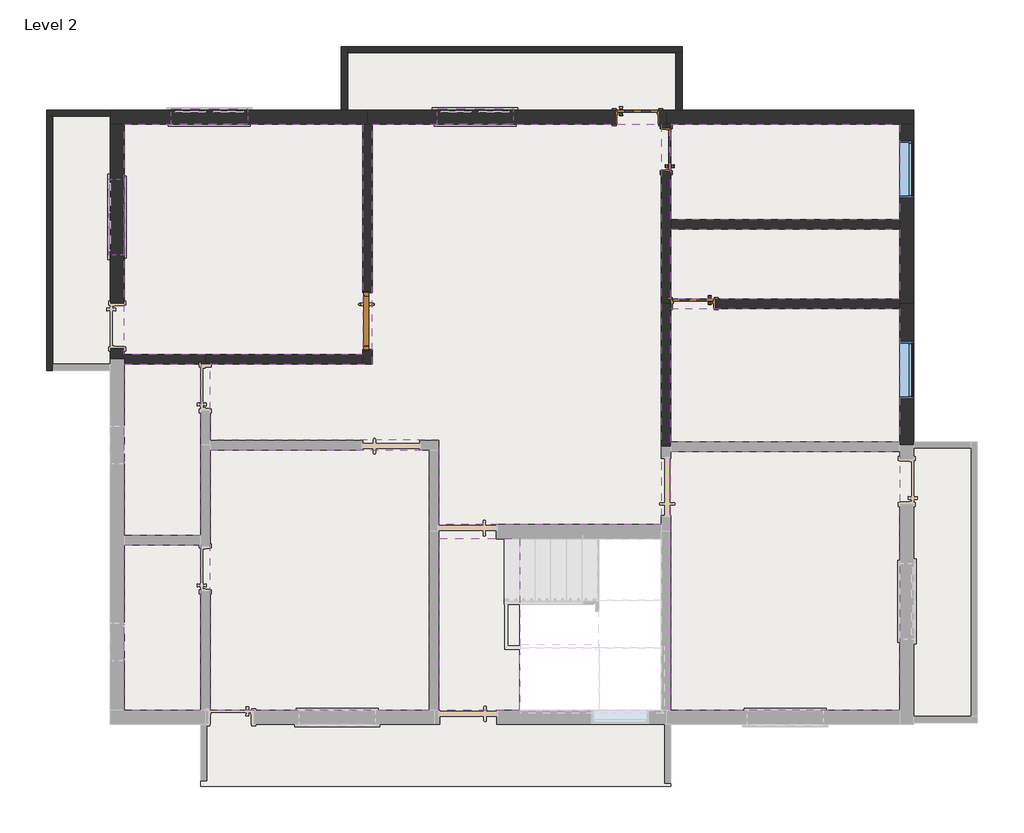
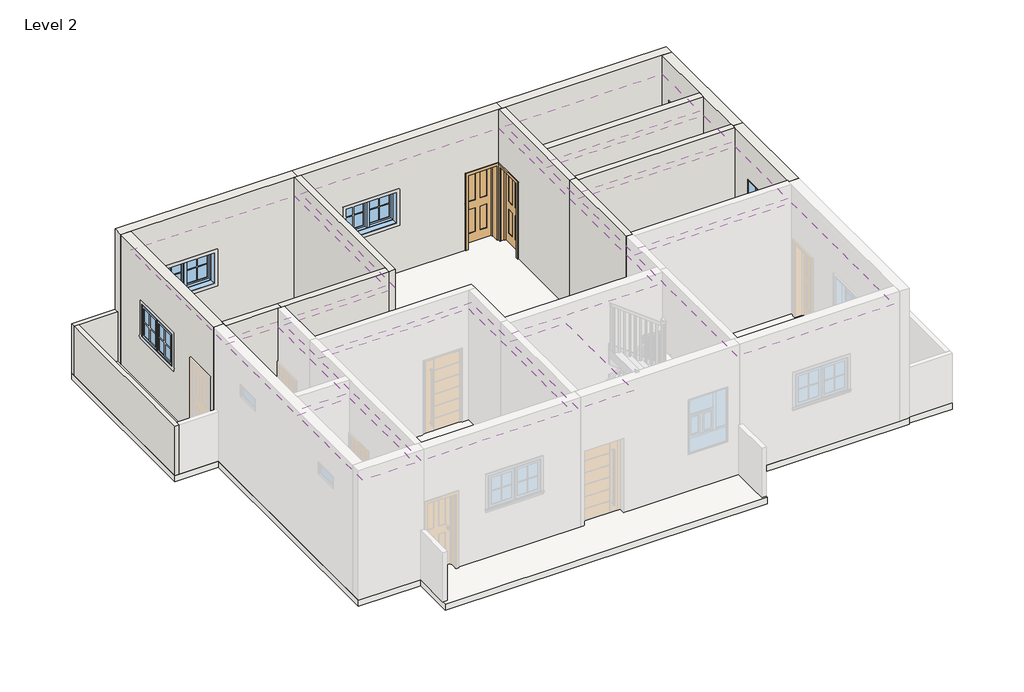
# One storey, part 2 of 3: 18 walls, 10 coverings, 5 windows, 4 doors, 1 slab.
"""IFC4 building model written with IfcOpenShell, lengths in millimetres."""

from ifc_helpers import new_model, si_unit, frame, origin, place, context, project, spatial, polyline, outline, extrude, faceted_brep, transform, mapped, element, save
from components import door_3_44036f4b, door_7109d6db, door_46909e31, m_window_awning_double_horizontal_4_8afcb0b2, m_window_casement_double_sash_variable_3_661e274a

model = new_model("IFC4")

# Units and contexts
model_context = context("Model", 3, world=origin())
ifc_project = project(units=[si_unit("LENGTHUNIT", "METRE", prefix="MILLI")], contexts=[model_context])

# Site, building, storey
site = spatial("IfcSite", under=ifc_project)
building = spatial("IfcBuilding", under=site)
storey = spatial("IfcBuildingStorey", under=building, Name="Level 2", Elevation=3200.4)

# Coverings
placement = place(None, origin())
element("IfcCovering", 1, ObjectType="Plain", at=placement, inside=storey, context=model_context, shape_type="SweptSolid", body=[
    extrude(outline(polyline([(-18062.7794909, 5121.4381491), (-14252.7794909, 5121.4381491), (-14252.7794909, 1438.4381491), (-16767.3794909, 1438.4381491), (-18062.7794909, 1438.4381491), (-18062.7794909, 5121.4381491)])), frame((0.0, 0.0, 5943.6), z_axis=(0.0, 0.0, 1.0), x_axis=(1.0, 0.0, 0.0)), (0.0, 0.0, 1.0), 57.0),
])
element("IfcCovering", 2, ObjectType="Plain", at=placement, inside=storey, context=model_context, shape_type="SweptSolid", body=[
    extrude(outline(polyline([(-16691.1794909, 1286.0381491), (-14100.3794909, 1286.0381491), (-14100.3794909, 5121.4381491), (-9477.5794909, 5121.4381491), (-9477.5794909, 2251.2381491), (-9477.5794909, -34.7618509), (-9477.5794909, -1279.3618509), (-13033.5794909, -1279.3618509), (-13033.5794909, 66.8381491), (-16691.1794909, 66.8381491), (-16691.1794909, 1286.0381491)])), frame((0.0, 0.0, 5943.6), z_axis=(0.0, 0.0, 1.0), x_axis=(1.0, 0.0, 0.0)), (0.0, 0.0, 1.0), 57.0),
])
element("IfcCovering", 3, ObjectType="Plain", at=placement, inside=storey, context=model_context, shape_type="SweptSolid", body=[
    extrude(outline(polyline([(-16843.5794909, -1457.1618509), (-18062.7794909, -1457.1618509), (-18062.7794909, 1286.0381491), (-16843.5794909, 1286.0381491), (-16843.5794909, -9.3618509), (-16843.5794909, -1457.1618509)])), frame((0.0, 0.0, 5943.6), z_axis=(0.0, 0.0, 1.0), x_axis=(1.0, 0.0, 0.0)), (0.0, 0.0, 1.0), 57.0),
])
element("IfcCovering", 4, ObjectType="Plain", at=placement, inside=storey, context=model_context, shape_type="SweptSolid", body=[
    extrude(outline(polyline([(-18062.7794909, -4251.1618509), (-18062.7794909, -1609.5618509), (-16843.5794909, -1609.5618509), (-16843.5794909, -4251.1618509), (-18062.7794909, -4251.1618509)])), frame((0.0, 0.0, 5943.6), z_axis=(0.0, 0.0, 1.0), x_axis=(1.0, 0.0, 0.0)), (0.0, 0.0, 1.0), 57.0),
])
element("IfcCovering", 5, ObjectType="Plain", at=placement, inside=storey, context=model_context, shape_type="SweptSolid", body=[
    extrude(outline(polyline([(-16691.1794909, -4251.1618509), (-16691.1794909, -85.5618509), (-13185.9794909, -85.5618509), (-13185.9794909, -1393.6618509), (-13185.9794909, -4251.1618509), (-16691.1794909, -4251.1618509)])), frame((0.0, 0.0, 5943.6), z_axis=(0.0, 0.0, 1.0), x_axis=(1.0, 0.0, 0.0)), (0.0, 0.0, 1.0), 57.0),
])
element("IfcCovering", 6, ObjectType="Plain", at=placement, inside=storey, context=model_context, shape_type="SweptSolid", body=[
    extrude(outline(polyline([(-13033.5794909, -4251.1618509), (-13033.5794909, -1507.9618509), (-11738.1794909, -1507.9618509), (-11738.1794909, -4251.1618509), (-13033.5794909, -4251.1618509)])), frame((0.0, 0.0, 5943.6), z_axis=(0.0, 0.0, 1.0), x_axis=(1.0, 0.0, 0.0)), (0.0, 0.0, 1.0), 57.0),
])
element("IfcCovering", 7, ObjectType="Plain", at=placement, inside=storey, context=model_context, shape_type="SweptSolid", body=[
    extrude(outline(polyline([(-5667.5794909, -4251.1618509), (-9325.1794909, -4251.1618509), (-9325.1794909, -1393.6618509), (-9325.1794909, -110.9618509), (-5667.5794909, -110.9618509), (-5667.5794909, -4251.1618509)])), frame((0.0, 0.0, 5943.6), z_axis=(0.0, 0.0, 1.0), x_axis=(1.0, 0.0, 0.0)), (0.0, 0.0, 1.0), 57.0),
])
element("IfcCovering", 8, ObjectType="Plain", at=placement, inside=storey, context=model_context, shape_type="SweptSolid", body=[
    extrude(outline(polyline([(-9325.1794909, 2175.0381491), (-5667.5794909, 2175.0381491), (-5667.5794909, 41.4381491), (-9325.1794909, 41.4381491), (-9325.1794909, 2175.0381491)])), frame((0.0, 0.0, 5943.6), z_axis=(0.0, 0.0, 1.0), x_axis=(1.0, 0.0, 0.0)), (0.0, 0.0, 1.0), 57.0),
])
element("IfcCovering", 9, ObjectType="Plain", at=placement, inside=storey, context=model_context, shape_type="SweptSolid", body=[
    extrude(outline(polyline([(-5667.5794909, 3445.0381491), (-5667.5794909, 2327.4381491), (-9325.1794909, 2327.4381491), (-9325.1794909, 3445.0381491), (-5667.5794909, 3445.0381491)])), frame((0.0, 0.0, 5943.6), z_axis=(0.0, 0.0, 1.0), x_axis=(1.0, 0.0, 0.0)), (0.0, 0.0, 1.0), 57.0),
])
element("IfcCovering", 10, ObjectType="Plain", at=placement, inside=storey, context=model_context, shape_type="SweptSolid", body=[
    extrude(outline(polyline([(-5667.5794909, 5121.4381491), (-5667.5794909, 3597.4381491), (-9325.1794909, 3597.4381491), (-9325.1794909, 5121.4381491), (-5667.5794909, 5121.4381491)])), frame((0.0, 0.0, 5943.6), z_axis=(0.0, 0.0, 1.0), x_axis=(1.0, 0.0, 0.0)), (0.0, 0.0, 1.0), 57.0),
])

# Doors
door_3_shape = door_3_44036f4b(model_context)
element("IfcDoor", 11, ObjectType="3'", at=placement, inside=storey, context=model_context, shape_type="MappedRepresentation", body=[
    mapped(door_3_shape, transform((-14176.5794909, 1971.8381491, 3200.4), x_axis=(0.0, -1.0, 0.0), y_axis=(1.0, 0.0, 0.0), z_axis=(0.0, 0.0, 1.0))),
])
door_shape = door_7109d6db(model_context)
element("IfcDoor", 12, ObjectType="M_Door-Interior-Single-4_Panel-Wood : 2'2\"", at=placement, inside=storey, context=model_context, shape_type="MappedRepresentation", body=[
    mapped(door_shape, transform((-9398.2044909, 4715.4381491, 3200.4), x_axis=(0.0, 1.0, 0.0), y_axis=(-1.0, 0.0, 0.0), z_axis=(0.0, 0.0, 1.0))),
])
element("IfcDoor", 13, ObjectType="M_Door-Interior-Single-4_Panel-Wood : 2'2\"", at=placement, inside=storey, context=model_context, shape_type="MappedRepresentation", body=[
    mapped(door_shape, transform((-8969.9794909, 2254.4131491, 3200.4), x_axis=(-1.0, 0.0, 0.0), y_axis=(0.0, -1.0, 0.0), z_axis=(0.0, 0.0, 1.0))),
])
door_2_shape = door_46909e31(model_context)
element("IfcDoor", 14, ObjectType="M_Door-Interior-Single-4_Panel-Wood : 2'2\"", at=placement, inside=storey, context=model_context, shape_type="MappedRepresentation", body=[
    mapped(door_2_shape, transform((-9858.1794909, 5238.9131491, 3200.4), x_axis=(1.0, 0.0, 0.0), y_axis=(0.0, 1.0, 0.0), z_axis=(0.0, 0.0, 1.0))),
])

# Slab
element("IfcSlab", 15, ObjectType="Generic 150mm", at=placement, inside=storey, context=model_context, shape_type="SweptSolid", body=[
    extrude(outline(polyline([(-18291.3794909, 1184.4381491), (-19307.3794909, 1184.4381491), (-19307.3794909, 5350.0381491), (-14596.2721539, 5350.0381491), (-14596.2721539, 6366.0381491), (-9142.3367869, 6366.0381491), (-9142.3367869, 5350.0381491), (-5438.9794909, 5350.0381491), (-5438.9794909, 41.4381491), (-4422.9794909, 41.4381491), (-4422.9794909, -4454.3618509), (-5438.9794909, -4454.3618509), (-5438.9794909, -4479.7618509), (-9325.1794909, -4479.7618509), (-9325.1794909, -5470.3618509), (-16843.5794909, -5470.3618509), (-16843.5794909, -4479.7618509), (-18291.3794909, -4479.7618509), (-18291.3794909, 1184.4381491)]), holes=[polyline([(-11738.1794909, -1507.9618509), (-11738.1794909, -4251.1618509), (-9477.5794909, -4251.1618509), (-9477.5794909, -1507.9618509), (-11738.1794909, -1507.9618509)])]), frame((0.0, 0.0, 3050.4), z_axis=(0.0, 0.0, 1.0), x_axis=(1.0, 0.0, 0.0)), (0.0, 0.0, 1.0), 150.0),
])

# Walls
element("IfcWall", 16, ObjectType="Generic - 4\"", at=placement, inside=storey, context=model_context, shape_type="Brep", body=[
    faceted_brep([(-14494.6721539, 5350.0381491, 3200.4), (-14494.6721539, 6264.4381491, 3200.4), (-14494.6721539, 6366.0381491, 3200.4), (-14494.6721539, 6366.0381491, 4419.6), (-14494.6721539, 6264.4381491, 4419.6), (-14494.6721539, 5350.0381491, 4419.6), (-14596.2721539, 5350.0381491, 3200.4), (-14596.2721539, 5350.0381491, 4419.6), (-14596.2721539, 6366.0381491, 4419.6), (-14596.2721539, 6366.0381491, 3200.4)], [[[0, 1, 2, 3, 4, 5]], [[6, 7, 8, 9]], [[2, 1, 0, 6, 9]], [[5, 4, 3, 8, 7]], [[0, 5, 7, 6]], [[3, 2, 9, 8]]]),
])
element("IfcWall", 17, ObjectType="Generic - 4\"", at=placement, inside=storey, context=model_context, shape_type="Brep", body=[
    faceted_brep([(-14494.6721539, 6264.4381491, 3200.4), (-9243.9367869, 6264.4381491, 3200.4), (-9142.3367869, 6264.4381491, 3200.4), (-9142.3367869, 6264.4381491, 4419.6), (-9243.9367869, 6264.4381491, 4419.6), (-14494.6721539, 6264.4381491, 4419.6), (-14494.6721539, 6366.0381491, 3200.4), (-14494.6721539, 6366.0381491, 4419.6), (-9142.3367869, 6366.0381491, 4419.6), (-9142.3367869, 6366.0381491, 3200.4)], [[[0, 1, 2, 3, 4, 5]], [[6, 7, 8, 9]], [[2, 1, 0, 6, 9]], [[5, 4, 3, 8, 7]], [[0, 5, 7, 6]], [[3, 2, 9, 8]]]),
])
element("IfcWall", 18, ObjectType="Generic - 4\"", at=placement, inside=storey, context=model_context, shape_type="SweptSolid", body=[
    extrude(outline(polyline([(-9243.9367869, 5350.0381491), (-9243.9367869, 6264.4381491), (-9142.3367869, 6264.4381491), (-9142.3367869, 5350.0381491), (-9243.9367869, 5350.0381491)])), frame((0.0, 0.0, 3200.4), z_axis=(0.0, 0.0, 1.0), x_axis=(1.0, 0.0, 0.0)), (0.0, 0.0, 1.0), 1219.2),
])
element("IfcWall", 19, ObjectType="Generic - 4\"", at=placement, inside=storey, context=model_context, shape_type="Brep", body=[
    faceted_brep([(-18291.3794909, 5350.0381491, 3200.4), (-19307.3794909, 5350.0381491, 3200.4), (-19307.3794909, 5350.0381491, 4419.6), (-18291.3794909, 5350.0381491, 4419.6), (-18291.3794909, 5248.4381491, 3200.4), (-18291.3794909, 5248.4381491, 4419.6), (-19205.7794909, 5248.4381491, 4419.6), (-19307.3794909, 5248.4381491, 4419.6), (-19307.3794909, 5248.4381491, 3200.4), (-19205.7794909, 5248.4381491, 3200.4)], [[[0, 1, 2, 3]], [[4, 5, 6, 7, 8, 9]], [[1, 0, 4, 9, 8]], [[3, 2, 7, 6, 5]], [[0, 3, 5, 4]], [[2, 1, 8, 7]]]),
])
element("IfcWall", 20, ObjectType="Generic - 4\"", at=placement, inside=storey, context=model_context, shape_type="Brep", body=[
    faceted_brep([(-19307.3794909, 5248.4381491, 3200.4), (-19307.3794909, 1184.4381491, 3200.4), (-19307.3794909, 1184.4381491, 4419.6), (-19307.3794909, 5248.4381491, 4419.6), (-19205.7794909, 5248.4381491, 3200.4), (-19205.7794909, 5248.4381491, 4419.6), (-19205.7794909, 1286.0381491, 4419.6), (-19205.7794909, 1184.4381491, 4419.6), (-19205.7794909, 1184.4381491, 3200.4), (-19205.7794909, 1286.0381491, 3200.4)], [[[0, 1, 2, 3]], [[4, 5, 6, 7, 8, 9]], [[1, 0, 4, 9, 8]], [[3, 2, 7, 6, 5]], [[0, 3, 5, 4]], [[2, 1, 8, 7]]]),
])
element("IfcWall", 21, ObjectType="Generic - 6\"", at=placement, inside=storey, context=model_context, shape_type="Brep", body=[
    faceted_brep([(-14252.7794909, 1286.0381491, 6400.8), (-14252.7794909, 1438.4381491, 6400.8), (-14252.7794909, 5121.4381491, 6400.8), (-14252.7794909, 5121.4381491, 3200.4), (-14252.7794909, 2429.0381491, 3200.4), (-14252.7794909, 2429.0381491, 5029.2), (-14252.7794909, 1514.6381491, 5029.2), (-14252.7794909, 1514.6381491, 3200.4), (-14252.7794909, 1438.4381491, 3200.4), (-14252.7794909, 1286.0381491, 3200.4), (-14100.3794909, 5121.4381491, 6400.8), (-14100.3794909, 1286.0381491, 6400.8), (-14100.3794909, 1286.0381491, 3200.4), (-14100.3794909, 1514.6381491, 3200.4), (-14100.3794909, 1514.6381491, 5029.2), (-14100.3794909, 2429.0381491, 5029.2), (-14100.3794909, 2429.0381491, 3200.4), (-14100.3794909, 5121.4381491, 3200.4), (-14232.7794909, 1514.6381491, 3200.4), (-14232.7794909, 1499.6381491, 3200.4), (-14155.7794909, 1499.6381491, 3200.4), (-14155.7794909, 1514.6381491, 3200.4), (-14176.5794909, 5121.4381491, 3200.4), (-14155.7794909, 2429.0381491, 3200.4), (-14155.7794909, 2444.0381491, 3200.4), (-14232.7794909, 2444.0381491, 3200.4), (-14232.7794909, 2429.0381491, 3200.4), (-14176.5794909, 5121.4381491, 6400.8), (-14232.7794909, 2429.0381491, 5029.2), (-14232.7794909, 1514.6381491, 5029.2), (-14155.7794909, 1514.6381491, 5029.2), (-14155.7794909, 2429.0381491, 5029.2), (-14232.7794909, 2444.0381491, 5044.2), (-14155.7794909, 2444.0381491, 5044.2), (-14155.7794909, 1499.6381491, 5044.2), (-14232.7794909, 1499.6381491, 5044.2)], [[[0, 1, 2, 3, 4, 5, 6, 7, 8, 9]], [[10, 11, 12, 13, 14, 15, 16, 17]], [[12, 9, 8, 7, 18, 19, 20, 21, 13]], [[3, 22, 17, 16, 23, 24, 25, 26, 4]], [[2, 1, 0, 11, 10, 27]], [[3, 2, 27, 10, 17, 22]], [[0, 9, 12, 11]], [[5, 28, 29, 6]], [[14, 30, 31, 15]], [[6, 29, 18, 7]], [[30, 14, 13, 21]], [[28, 5, 4, 26]], [[15, 31, 23, 16]], [[32, 33, 34, 35]], [[35, 34, 20, 19]], [[31, 30, 21, 20, 34, 33, 24, 23]], [[33, 32, 25, 24]], [[29, 28, 26, 25, 32, 35, 19, 18]]]),
])
element("IfcWall", 22, ObjectType="Generic - 6\"", at=placement, inside=storey, context=model_context, shape_type="Brep", body=[
    faceted_brep([(-14252.7794909, 1438.4381491, 3200.4), (-16767.3794909, 1438.4381491, 3200.4), (-16767.3794909, 1438.4381491, 6400.8), (-14252.7794909, 1438.4381491, 6400.8), (-14252.7794909, 1286.0381491, 3200.4), (-14252.7794909, 1286.0381491, 6400.8), (-16691.1794909, 1286.0381491, 6400.8), (-16767.3794909, 1286.0381491, 6400.8), (-16767.3794909, 1286.0381491, 3200.4), (-16691.1794909, 1286.0381491, 3200.4)], [[[0, 1, 2, 3]], [[4, 5, 6, 7, 8, 9]], [[1, 0, 4, 9, 8]], [[2, 1, 8, 7]], [[3, 2, 7, 6, 5]], [[0, 3, 5, 4]]]),
])
element("IfcWall", 23, ObjectType="Generic - 6\"", at=placement, inside=storey, context=model_context, shape_type="SweptSolid", body=[
    extrude(outline(polyline([(-5667.5794909, 3445.0381491), (-9325.1794909, 3445.0381491), (-9325.1794909, 3597.4381491), (-5667.5794909, 3597.4381491), (-5667.5794909, 3445.0381491)])), frame((0.0, 0.0, 3200.4), z_axis=(0.0, 0.0, 1.0), x_axis=(1.0, 0.0, 0.0)), (0.0, 0.0, 1.0), 3200.4),
])
element("IfcWall", 24, ObjectType="Generic - 6\"", at=placement, inside=storey, context=model_context, shape_type="Brep", body=[
    faceted_brep([(-9325.1794909, 2327.4381491, 6400.8), (-5667.5794909, 2327.4381491, 6400.8), (-5667.5794909, 2327.4381491, 3200.4), (-8614.7794909, 2327.4381491, 3200.4), (-8614.7794909, 2327.4381491, 5054.2), (-9325.1794909, 2327.4381491, 5054.2), (-5667.5794909, 2175.0381491, 6400.8), (-9325.1794909, 2175.0381491, 6400.8), (-9325.1794909, 2175.0381491, 5054.2), (-8614.7794909, 2175.0381491, 5054.2), (-8614.7794909, 2175.0381491, 3200.4), (-5667.5794909, 2175.0381491, 3200.4), (-5667.5794909, 2251.2381491, 3200.4), (-9325.1794909, 2251.2381491, 6400.8), (-5667.5794909, 2251.2381491, 6400.8)], [[[0, 1, 2, 3, 4, 5]], [[6, 7, 8, 9, 10, 11]], [[2, 12, 11, 10, 3]], [[1, 0, 13, 7, 6, 14]], [[2, 1, 14, 6, 11, 12]], [[7, 13, 0, 5, 8]], [[4, 9, 8, 5]], [[9, 4, 3, 10]]]),
])
element("IfcWall", 25, ObjectType="Generic - 6\"", at=placement, inside=storey, context=model_context, shape_type="Brep", body=[
    faceted_brep([(-9325.1794909, 5121.4381491, 6400.8), (-9325.1794909, 3597.4381491, 6400.8), (-9325.1794909, 3445.0381491, 6400.8), (-9325.1794909, 2327.4381491, 6400.8), (-9325.1794909, 2251.2381491, 6400.8), (-9325.1794909, 2251.2381491, 3200.4), (-9325.1794909, 3445.0381491, 3200.4), (-9325.1794909, 3597.4381491, 3200.4), (-9325.1794909, 4360.2381491, 3200.4), (-9325.1794909, 4360.2381491, 5054.2), (-9325.1794909, 5070.6381491, 5054.2), (-9325.1794909, 5070.6381491, 3200.4), (-9325.1794909, 5121.4381491, 3200.4), (-9477.5794909, 2251.2381491, 6400.8), (-9477.5794909, 5121.4381491, 6400.8), (-9477.5794909, 5121.4381491, 3200.4), (-9477.5794909, 5070.6381491, 3200.4), (-9477.5794909, 5070.6381491, 5054.2), (-9477.5794909, 4360.2381491, 5054.2), (-9477.5794909, 4360.2381491, 3200.4), (-9477.5794909, 2251.2381491, 3200.4), (-9401.3794909, 5121.4381491, 3200.4), (-9401.3794909, 5121.4381491, 6400.8)], [[[0, 1, 2, 3, 4, 5, 6, 7, 8, 9, 10, 11, 12]], [[13, 14, 15, 16, 17, 18, 19, 20]], [[15, 21, 12, 11, 16]], [[5, 20, 19, 8, 7, 6]], [[4, 3, 2, 1, 0, 22, 14, 13]], [[5, 4, 13, 20]], [[0, 12, 21, 15, 14, 22]], [[10, 17, 16, 11]], [[17, 10, 9, 18]], [[18, 9, 8, 19]]]),
])
element("IfcWall", 26, ObjectType="Generic - 6\"", at=placement, inside=storey, context=model_context, shape_type="Brep", body=[
    faceted_brep([(-9325.1794909, -34.7618509, 3200.4), (-9325.1794909, 41.4381491, 3200.4), (-9325.1794909, 2251.2381491, 3200.4), (-9325.1794909, 2251.2381491, 6400.8), (-9325.1794909, 2175.0381491, 6400.8), (-9325.1794909, 41.4381491, 6400.8), (-9325.1794909, -34.7618509, 6400.8), (-9477.5794909, -34.7618509, 3200.4), (-9477.5794909, -34.7618509, 6400.8), (-9477.5794909, 2251.2381491, 6400.8), (-9477.5794909, 2251.2381491, 3200.4)], [[[0, 1, 2, 3, 4, 5, 6]], [[7, 8, 9, 10]], [[2, 1, 0, 7, 10]], [[3, 2, 10, 9]], [[6, 5, 4, 3, 9, 8]], [[0, 6, 8, 7]]]),
])
element("IfcWall", 27, ObjectType="Generic - 6\"", at=placement, inside=storey, context=model_context, shape_type="Brep", body=[
    faceted_brep([(-16767.3794909, 1438.4381491, 3200.4), (-18062.7794909, 1438.4381491, 3200.4), (-18062.7794909, 1438.4381491, 6400.8), (-16767.3794909, 1438.4381491, 6400.8), (-16767.3794909, 1286.0381491, 3200.4), (-16767.3794909, 1286.0381491, 6400.8), (-16843.5794909, 1286.0381491, 6400.8), (-18062.7794909, 1286.0381491, 6400.8), (-18062.7794909, 1286.0381491, 3200.4), (-16843.5794909, 1286.0381491, 3200.4), (-18062.7794909, 1362.2381491, 3200.4), (-18062.7794909, 1362.2381491, 6400.8)], [[[0, 1, 2, 3]], [[4, 5, 6, 7, 8, 9]], [[1, 0, 4, 9, 8, 10]], [[3, 2, 11, 7, 6, 5]], [[0, 3, 5, 4]], [[2, 1, 10, 8, 7, 11]]]),
])
element("IfcWall", 28, ObjectType="Generic - 9\"", at=placement, inside=storey, context=model_context, shape_type="Brep", body=[
    faceted_brep([(-18291.3794909, 5121.4381491, 6400.8), (-18291.3794909, 5121.4381491, 3200.4), (-18062.7794909, 5121.4381491, 3200.4), (-14252.7794909, 5121.4381491, 3200.4), (-14176.5794909, 5121.4381491, 3200.4), (-14176.5794909, 5121.4381491, 6400.8), (-14252.7794909, 5121.4381491, 6400.8), (-18062.7794909, 5121.4381491, 6400.8), (-16094.2794909, 5121.4381491, 5219.6), (-16094.2794909, 5121.4381491, 4419.6), (-17313.4794909, 5121.4381491, 4419.6), (-17313.4794909, 5121.4381491, 5219.6), (-18291.3794909, 5350.0381491, 3200.4), (-18291.3794909, 5350.0381491, 4419.6), (-18291.3794909, 5350.0381491, 6400.8), (-14176.5794909, 5350.0381491, 6400.8), (-14176.5794909, 5350.0381491, 3200.4), (-14494.6721539, 5350.0381491, 3200.4), (-14596.2721539, 5350.0381491, 3200.4), (-16094.2794909, 5350.0381491, 5219.6), (-17313.4794909, 5350.0381491, 5219.6), (-17313.4794909, 5350.0381491, 4419.6), (-16094.2794909, 5350.0381491, 4419.6), (-18291.3794909, 5248.4381491, 3200.4)], [[[0, 1, 2, 3, 4, 5, 6, 7], [8, 9, 10, 11]], [[12, 13, 14, 15, 16, 17, 18], [19, 20, 21, 22]], [[4, 3, 2, 1, 23, 12, 18, 17, 16]], [[5, 4, 16, 15]], [[0, 7, 6, 5, 15, 14]], [[0, 14, 13, 12, 23, 1]], [[9, 8, 19, 22]], [[10, 9, 22, 21]], [[11, 10, 21, 20]], [[8, 11, 20, 19]]]),
])
element("IfcWall", 29, ObjectType="Generic - 9\"", at=placement, inside=storey, context=model_context, shape_type="Brep", body=[
    faceted_brep([(-5667.5794909, 5121.4381491, 3200.4), (-5667.5794909, 3597.4381491, 3200.4), (-5667.5794909, 3445.0381491, 3200.4), (-5667.5794909, 2327.4381491, 3200.4), (-5667.5794909, 2251.2381491, 3200.4), (-5667.5794909, 2251.2381491, 6400.8), (-5667.5794909, 2327.4381491, 6400.8), (-5667.5794909, 3445.0381491, 6400.8), (-5667.5794909, 3597.4381491, 6400.8), (-5667.5794909, 5121.4381491, 6400.8), (-5667.5794909, 3943.5131491, 5450.4), (-5667.5794909, 3943.5131491, 4100.4), (-5667.5794909, 4857.9131491, 4100.4), (-5667.5794909, 4857.9131491, 5450.4), (-5438.9794909, 5121.4381491, 3200.4), (-5438.9794909, 5121.4381491, 6400.8), (-5438.9794909, 2251.2381491, 6400.8), (-5438.9794909, 2251.2381491, 3200.4), (-5438.9794909, 3943.5131491, 5450.4), (-5438.9794909, 4857.9131491, 5450.4), (-5438.9794909, 4857.9131491, 4100.4), (-5438.9794909, 3943.5131491, 4100.4)], [[[0, 1, 2, 3, 4, 5, 6, 7, 8, 9], [10, 11, 12, 13]], [[14, 15, 16, 17], [18, 19, 20, 21]], [[4, 3, 2, 1, 0, 14, 17]], [[5, 4, 17, 16]], [[9, 8, 7, 6, 5, 16, 15]], [[0, 9, 15, 14]], [[11, 10, 18, 21]], [[12, 11, 21, 20]], [[13, 12, 20, 19]], [[10, 13, 19, 18]]]),
])
element("IfcWall", 30, ObjectType="Generic - 9\"", at=placement, inside=storey, context=model_context, shape_type="Brep", body=[
    faceted_brep([(-9401.3794909, 5121.4381491, 3200.4), (-9401.3794909, 5121.4381491, 6400.8), (-9477.5794909, 5121.4381491, 6400.8), (-14100.3794909, 5121.4381491, 6400.8), (-14176.5794909, 5121.4381491, 6400.8), (-14176.5794909, 5121.4381491, 3200.4), (-14100.3794909, 5121.4381491, 3200.4), (-10213.3794909, 5121.4381491, 3200.4), (-10213.3794909, 5121.4381491, 5054.2), (-9502.9794909, 5121.4381491, 5054.2), (-9502.9794909, 5121.4381491, 3200.4), (-9477.5794909, 5121.4381491, 3200.4), (-11844.5419909, 5121.4381491, 5219.6), (-11844.5419909, 5121.4381491, 4419.6), (-13063.7419909, 5121.4381491, 4419.6), (-13063.7419909, 5121.4381491, 5219.6), (-9401.3794909, 5350.0381491, 6400.8), (-9401.3794909, 5350.0381491, 3200.4), (-9502.9794909, 5350.0381491, 3200.4), (-9502.9794909, 5350.0381491, 5054.2), (-10213.3794909, 5350.0381491, 5054.2), (-10213.3794909, 5350.0381491, 3200.4), (-14176.5794909, 5350.0381491, 3200.4), (-14176.5794909, 5350.0381491, 6400.8), (-11844.5419909, 5350.0381491, 5219.6), (-13063.7419909, 5350.0381491, 5219.6), (-13063.7419909, 5350.0381491, 4419.6), (-11844.5419909, 5350.0381491, 4419.6)], [[[0, 1, 2, 3, 4, 5, 6, 7, 8, 9, 10, 11], [12, 13, 14, 15]], [[16, 17, 18, 19, 20, 21, 22, 23], [24, 25, 26, 27]], [[5, 22, 21, 7, 6]], [[17, 0, 11, 10, 18]], [[1, 0, 17, 16]], [[4, 3, 2, 1, 16, 23]], [[5, 4, 23, 22]], [[12, 15, 25, 24]], [[15, 14, 26, 25]], [[14, 13, 27, 26]], [[13, 12, 24, 27]], [[9, 19, 18, 10]], [[19, 9, 8, 20]], [[20, 8, 7, 21]]]),
])
element("IfcWall", 31, ObjectType="Generic - 9\"", at=placement, inside=storey, context=model_context, shape_type="Brep", body=[
    faceted_brep([(-9401.3794909, 5121.4381491, 3200.4), (-9325.1794909, 5121.4381491, 3200.4), (-5667.5794909, 5121.4381491, 3200.4), (-5438.9794909, 5121.4381491, 3200.4), (-5438.9794909, 5121.4381491, 6400.8), (-5667.5794909, 5121.4381491, 6400.8), (-9325.1794909, 5121.4381491, 6400.8), (-9401.3794909, 5121.4381491, 6400.8), (-9401.3794909, 5350.0381491, 3200.4), (-9401.3794909, 5350.0381491, 6400.8), (-5438.9794909, 5350.0381491, 6400.8), (-5438.9794909, 5350.0381491, 3200.4), (-9142.3367869, 5350.0381491, 3200.4), (-9243.9367869, 5350.0381491, 3200.4)], [[[0, 1, 2, 3, 4, 5, 6, 7]], [[8, 9, 10, 11, 12, 13]], [[3, 2, 1, 0, 8, 13, 12, 11]], [[7, 6, 5, 4, 10, 9]], [[0, 7, 9, 8]], [[4, 3, 11, 10]]]),
])
element("IfcWall", 32, ObjectType="Generic - 9\"", at=placement, inside=storey, context=model_context, shape_type="Brep", body=[
    faceted_brep([(-5667.5794909, 2251.2381491, 3200.4), (-5667.5794909, 2175.0381491, 3200.4), (-5667.5794909, -9.3618509, 3200.4), (-5667.5794909, -9.3618509, 6400.8), (-5667.5794909, 2175.0381491, 6400.8), (-5667.5794909, 2251.2381491, 6400.8), (-5667.5794909, 732.0006491, 5450.4), (-5667.5794909, 732.0006491, 4100.4), (-5667.5794909, 1646.4006491, 4100.4), (-5667.5794909, 1646.4006491, 5450.4), (-5438.9794909, 2251.2381491, 3200.4), (-5438.9794909, 2251.2381491, 6400.8), (-5438.9794909, -9.3618509, 6400.8), (-5438.9794909, -9.3618509, 3200.4), (-5438.9794909, 41.4381491, 3200.4), (-5438.9794909, 732.0006491, 5450.4), (-5438.9794909, 1646.4006491, 5450.4), (-5438.9794909, 1646.4006491, 4100.4), (-5438.9794909, 732.0006491, 4100.4)], [[[0, 1, 2, 3, 4, 5], [6, 7, 8, 9]], [[10, 11, 12, 13, 14], [15, 16, 17, 18]], [[2, 1, 0, 10, 14, 13]], [[5, 4, 3, 12, 11]], [[0, 5, 11, 10]], [[6, 9, 16, 15]], [[9, 8, 17, 16]], [[8, 7, 18, 17]], [[7, 6, 15, 18]], [[2, 13, 12, 3]]]),
])
element("IfcWall", 33, ObjectType="Generic - 9\"", at=placement, inside=storey, context=model_context, shape_type="Brep", body=[
    faceted_brep([(-18062.7794909, 5121.4381491, 6400.8), (-18062.7794909, 1438.4381491, 6400.8), (-18062.7794909, 1362.2381491, 6400.8), (-18062.7794909, 1362.2381491, 3200.4), (-18062.7794909, 1438.4381491, 3200.4), (-18062.7794909, 1540.0381491, 3200.4), (-18062.7794909, 1540.0381491, 5054.2), (-18062.7794909, 2250.4381491, 5054.2), (-18062.7794909, 2250.4381491, 3200.4), (-18062.7794909, 5121.4381491, 3200.4), (-18062.7794909, 4247.5131491, 5219.6), (-18062.7794909, 4247.5131491, 4419.6), (-18062.7794909, 3028.3131491, 4419.6), (-18062.7794909, 3028.3131491, 5219.6), (-18291.3794909, 1362.2381491, 6400.8), (-18291.3794909, 5121.4381491, 6400.8), (-18291.3794909, 5121.4381491, 3200.4), (-18291.3794909, 2250.4381491, 3200.4), (-18291.3794909, 2250.4381491, 5054.2), (-18291.3794909, 1540.0381491, 5054.2), (-18291.3794909, 1540.0381491, 3200.4), (-18291.3794909, 1362.2381491, 3200.4), (-18291.3794909, 4247.5131491, 5219.6), (-18291.3794909, 3028.3131491, 5219.6), (-18291.3794909, 3028.3131491, 4419.6), (-18291.3794909, 4247.5131491, 4419.6)], [[[0, 1, 2, 3, 4, 5, 6, 7, 8, 9], [10, 11, 12, 13]], [[14, 15, 16, 17, 18, 19, 20, 21], [22, 23, 24, 25]], [[16, 9, 8, 17]], [[3, 21, 20, 5, 4]], [[2, 1, 0, 15, 14]], [[3, 2, 14, 21]], [[9, 16, 15, 0]], [[10, 13, 23, 22]], [[13, 12, 24, 23]], [[12, 11, 25, 24]], [[11, 10, 22, 25]], [[19, 6, 5, 20]], [[6, 19, 18, 7]], [[7, 18, 17, 8]]]),
])

# Windows
m_window_awning_double_horizontal_4_shape = m_window_awning_double_horizontal_4_8afcb0b2(model_context)
element("IfcWindow", 34, ObjectType="M_Window-Awning-Double-Horizontal : 4'", at=placement, inside=storey, context=model_context, shape_type="MappedRepresentation", body=[
    mapped(m_window_awning_double_horizontal_4_shape, transform((-16703.8794909, 5235.7381491, 3519.6), x_axis=(1.0, 0.0, 0.0), y_axis=(0.0, 1.0, 0.0), z_axis=(0.0, 0.0, 1.0))),
])
element("IfcWindow", 35, ObjectType="M_Window-Awning-Double-Horizontal : 4'", at=placement, inside=storey, context=model_context, shape_type="MappedRepresentation", body=[
    mapped(m_window_awning_double_horizontal_4_shape, transform((-18177.0794909, 3637.9131491, 3519.6), x_axis=(0.0, 1.0, 0.0), y_axis=(-1.0, 0.0, 0.0), z_axis=(0.0, 0.0, 1.0))),
])
element("IfcWindow", 36, ObjectType="M_Window-Awning-Double-Horizontal : 4'", at=placement, inside=storey, context=model_context, shape_type="MappedRepresentation", body=[
    mapped(m_window_awning_double_horizontal_4_shape, transform((-12454.1419909, 5235.7381491, 3519.6), x_axis=(1.0, 0.0, 0.0), y_axis=(0.0, 1.0, 0.0), z_axis=(0.0, 0.0, 1.0))),
])
m_window_casement_double_sash_variable_3_shape = m_window_casement_double_sash_variable_3_661e274a(model_context)
element("IfcWindow", 37, ObjectType="M_Window-Casement-Double-Sash-Variable : 3'", at=placement, inside=storey, context=model_context, shape_type="MappedRepresentation", body=[
    mapped(m_window_casement_double_sash_variable_3_shape, transform((-5553.2794909, 1189.2006491, 3200.4), x_axis=(0.0, -1.0, 0.0), y_axis=(1.0, 0.0, 0.0), z_axis=(0.0, 0.0, 1.0))),
])
element("IfcWindow", 38, ObjectType="M_Window-Casement-Double-Sash-Variable : 3'", at=placement, inside=storey, context=model_context, shape_type="MappedRepresentation", body=[
    mapped(m_window_casement_double_sash_variable_3_shape, transform((-5553.2794909, 4400.7131491, 3200.4), x_axis=(0.0, -1.0, 0.0), y_axis=(1.0, 0.0, 0.0), z_axis=(0.0, 0.0, 1.0))),
])

save(model, "model.ifc")

# Revit data of these elements
# Type "Plain"
#   built-in parameter 1002203 = 1 (stored number, unit not read)
#   built-in parameter 1002202 = 1 (stored number, unit not read)
#   Layers, outside or top first: 0' - 1.77165" "Metal Stud Layer" (function 1); 0' - 0.47244" "Gypsum Wall Board" (function 1)
# Type "3'"
#   Type Mark = "41"
#   Water resistance = "up to Class E900, EN 12208:2001"
#   Uniclass2015Version = "v1.21"
#   Uniclass2015Reference = "Ss_25_30_20_30"
#   Uniclass2015Description = "Frame and door leaf system"
#   URL = "www.aluprof.com"
#   Type IFC Predefined Type = "USERDEFINED"
#   Right-hand / Left-hand door [instance default] = ""
#   Resistance to wind load = "up to Class C5/B5, EN 12210:2001"
#   Insert type = "ST"
#   Hardware [instance default] = ""
#   Product page = "https://aluprof.com/en/architects/offer/window-and-door-systems/panel-doors#visualisation"
#   Operation = "SinglePanelOutwardOpening"
#   Opening type = "Outward"
#   NBSReference = "25-50-20/125"
#   NBSDescription = "Frame and door leaf system"
#   Important = "The actual acceptable construction dimensions are dependent on the selection of profiles and hardware, glazing type, construction weight and the construction’s operating conditions. These should be determined by a suitably qualified person, and using ALUPROF’s calculation software"
#   IfcExportType = "USERDEFINED"
#   IfcExportAs = "IfcDoorType"
#   Handle type [instance default] = ""
#   Manufacturer = "ALUPROF SA"
#   Export Type to IFC As = "IfcDoorType"
#   Door sill type [instance default] = ""
#   Description = "External single-leaf panel door outward opening"
#   Model = "MB-86 ST Panel Door AD07"
#   Content of the recyclate in the material = "69.2%"
#   COBie.Type.WarrantyDurationParts = ""
#   COBie.Type.Name = ""
#   COBie.Type.Manufacturer = "ALUPROF SA"
#   COBie.Space.Name = ""
#   COBie.Floor.Name = ""
#   COBie.Facility.Name = ""
#   COBie.CreatedOn = ""
#   COBie.Component.WarrantyStartDate = ""
#   COBie.Component.Name = "MB-86 ST Panel Door AD07"
#   Burglar resistance = "RC2"
#   Air permeability = "up to Class 4, EN 12207:2001"
#   Width of the active leaf = 2' - 8.17717"
#   Placement in wall = 0' - 0.7874"
#   Thickness = 0' - 3.0315"
#   Height of the opening sash = 5' - 9.44094"
#   Handle Offset = 3' - 5.33858"
#   Rough Height = 6' - 2.40945"
#   Rough Width = 3' - 1.1811"
#   Height = 6' - 0"
#   Width = 3' - 0"
#   Construction depth = 0' - 3.0315"
#   Clear opening width = 2' - 3.94882"
#   Clear opening height = 5' - 8.47638"
#   Height of the array = 0' - 11.08136"
#   Schedule No. [instance default] = 1
#   Handrail [instance default] = yes
#   IsExternal = yes
#   Handle [instance default] = no
#   Door closer [instance default] = no
#   Function = 1
#   COBie.Type = yes
#   COBie = yes
#   Access control [instance default] = no
#   Panel = element 361060
#   Wall Closure = (empty or 0)
# Type "M_Door-Interior-Single-4_Panel-Wood : 2'2\""
#   Type Mark = "43"
#   Assembly Code = "C1020300"
#   Analytic Construction = "Wooden"
#   Top Rail = 0' - 4.72441"
#   Thickness = 0' - 1.37795"
#   Thermal Resistance (R) = 0.455703 (m²·K)/W
#   Swing Angle [instance default] = 90.00°
#   Stiles = 0' - 4.72441"
#   Rough Width = 2' - 3.9685"
#   Rough Height = 6' - 0.98425"
#   Mullion = 0' - 4.52756"
#   Lock Rail = 0' - 7.87402"
#   Height = 6' - 0"
#   Width = 2' - 2"
#   Heat Transfer Coefficient (U) = 2.19465 W/(m²·K)
#   Bottom Rail = 0' - 9.05512"
#   Trim Material = Cherry
#   Panel Material = Cherry
#   Frame Material = Cherry
#   Door Handle Material = Aluminum
#   Visual Light Transmittance = 0
#   Solar Heat Gain Coefficient = 0
#   Wall Closure = (empty or 0)
#   Function = (empty or 0)
# Type "Generic 150mm"
#   Function = 0
#   Layers, outside or top first: 0' - 5.90551" no material (function 1)
# Type "Generic - 4\""
#   Layers, outside or top first: 0' - 4" no material (function 1)
# Type "Generic - 6\""
#   Layers, outside or top first: 0' - 6" no material (function 1)
# Type "Generic - 9\""
#   Layers, outside or top first: 0' - 9" no material (function 1)
# Type "M_Window-Awning-Double-Horizontal : 4'"
#   Type Mark = "28"
#   Fire Rating = "0.5h"
#   Assembly Code = "B2020100"
#   Analytic Construction = "Double glazing - domestic"
#   Window Inset [instance default] = 0' - 0"
#   Wall Thickness [instance default] = 0' - 5.90551"
#   Interior Wall Closure [instance default] = 0' - 2.15551"
#   Half Width = 2' - 0"
#   Visual Light Transmittance = 0.81
#   Thermal Resistance (R) = 0.319569 (m²·K)/W
#   Solar Heat Gain Coefficient = 0.76
#   Rough Width = 4' - 0.59055"
#   Rough Height = 2' - 8.08661"
#   Height = 2' - 7.49606"
#   Heat Transfer Coefficient (U) = 3.12929 W/(m²·K)
#   Frame Extension [instance default] = 0' - 0 1/4"
#   Exterior Wall Closure [instance default] = 0' - 1 1/4"
#   Extension Jamb [instance default] = 0' - 2.15551"
#   Default Sill Height = 2' - 11.43307"
#   Width = 4' - 0"
#   Muntin Visibility = yes
#   Interior Trim Visibility [instance default] = yes
#   Exterior Trim Visibility [instance default] = yes
#   Extension Jamb Visibility [instance default] = yes
#   Interior Trim Material = Wood - Stained
#   Muntin Pattern = M_Muntin Pattern_2x2 : M_Muntin Pattern_2x2
#   Interior Trim = M_Trim-Window-Interior-Flat : Picture Frame
#   Interior Frame Material = Wood - Stained
#   Glass Panel Material = Glass
#   Exterior Trim Material = Clad - White
#   Exterior Trim = M_Trim-Window-Exterior-Flat : with Sill
#   Exterior Frame Material = Clad - White
#   Wall Closure = (empty or 0)
# Type "M_Window-Casement-Double-Sash-Variable : 3'"
#   Type Mark = "36"
#   Fire Rating = "0.5h"
#   Assembly Code = "B2020100"
#   Analytic Construction = "Double glazing - domestic"
#   Window Inset [instance default] = 0' - 0 5/8"
#   Wall Thickness [instance default] = 0' - 5.90551"
#   Visual Light Transmittance = 0.81
#   Transom Height Ratio = 0.3
#   Transom Height = 1' - 3.94488"
#   Thermal Resistance (R) = 0.319569 (m²·K)/W
#   Solar Heat Gain Coefficient = 0.76
#   Rough Width = 3' - 0.59055"
#   Rough Height = 4' - 5.74016"
#   Opening Window Height = 1' - 9.25984"
#   Heat Transfer Coefficient (U) = 3.12929 W/(m²·K)
#   Height = 4' - 5.14961"
#   Frame Gap 3 [instance default] = 0' - 1.65041"
#   Frame Gap 2 [instance default] = 0' - 0.62598"
#   Frame Gap 1 = 0' - 1 51/128"
#   Window Width = 1' - 0"
#   Default Sill Height = 2' - 11.43307"
#   Width = 3' - 0"
#   Frame Material = Metal - Aluminum
#   Glass Panel Material = Glass
#   Wall Closure = (empty or 0)
# Elements 1, 2, 3, 4, 5, 6, 7, 8, 9, 10 (IfcCovering, "Plain")
#   Height Offset From Level = 9' - 0"
#   Phase Created = New Construction
#   Materials on its faces: "Gypsum Wall Board", "Metal Stud Layer"
# Element 11 (IfcDoor, "3'")
#   Right-hand / Left-hand door = ""
#   Hardware = ""
#   Handle type = ""
#   Door sill type = ""
#   Schedule No. = 1
#   Handrail = yes
#   Handle = no
#   Door closer = no
#   Access control = no
#   Phase Created = New Construction
# Elements 12, 13, 14 (IfcDoor, "M_Door-Interior-Single-4_Panel-Wood : 2'2\"")
#   Swing Angle = 90.00°
#   Phase Created = New Construction
#   Materials on its faces: "Cherry", "Aluminum"
# Element 15 (IfcSlab, "Generic 150mm")
#   Height Offset From Level = 0' - 0"
#   Phase Created = New Construction
#   Materials on its faces: "WALL2", "Default Floor", "FLOORING TILES 1"
# Elements 16, 17, 18 (IfcWall, "Generic - 4\"")
#   Top Offset = 0' - 0"
#   Base Offset = 0' - 0"
#   Unconnected Height = 4' - 0"
#   wall height = 4' - 0"
#   Phase Created = New Construction
#   Base Constraint = Level 2
#   Materials on its faces: "Default Wall", "WALL2"
# Elements 19, 20 (IfcWall, "Generic - 4\"")
#   Top Offset = 0' - 0"
#   Base Offset = 0' - 0"
#   Unconnected Height = 4' - 0"
#   wall height = 4' - 0"
#   Phase Created = New Construction
#   Base Constraint = Level 2
#   Materials on its faces: "WALL2", "Default Wall"
# Element 21 (IfcWall, "Generic - 6\"")
#   Top Offset = 0' - 0"
#   Base Offset = 0' - 0"
#   Unconnected Height = 10' - 6"
#   wall height = 10' - 6"
#   Phase Created = New Construction
#   Base Constraint = Level 2
#   Materials on its faces: "Default Wall", "LIVING 2", "BED ROOM WALL1"
# Element 22 (IfcWall, "Generic - 6\"")
#   Top Offset = 0' - 0"
#   Base Offset = 0' - 0"
#   Unconnected Height = 10' - 6"
#   wall height = 10' - 6"
#   Phase Created = New Construction
#   Base Constraint = Level 2
#   Materials on its faces: "Default Wall", "BED ROOM WALL 2", "LIVING 2"
# Element 23 (IfcWall, "Generic - 6\"")
#   Top Offset = 0' - 0"
#   Base Offset = 0' - 0"
#   Unconnected Height = 10' - 6"
#   wall height = 10' - 6"
#   Phase Created = New Construction
#   Base Constraint = Level 2
#   Materials on its faces: "Default Wall", "BED ROOM WALL 3", "BED ROOM WALL1"
# Elements 24, 25 (IfcWall, "Generic - 6\"")
#   Top Offset = 0' - 0"
#   Base Offset = 0' - 0"
#   Unconnected Height = 10' - 6"
#   wall height = 10' - 6"
#   Phase Created = New Construction
#   Base Constraint = Level 2
#   Materials on its faces: "Default Wall", "BED ROOM WALL1", "LIVING 2"
# Element 26 (IfcWall, "Generic - 6\"")
#   Top Offset = 0' - 0"
#   Base Offset = 0' - 0"
#   Unconnected Height = 10' - 6"
#   wall height = 10' - 6"
#   Phase Created = New Construction
#   Base Constraint = Level 2
#   Materials on its faces: "Default Wall", "LIVING", "LIVING 2"
# Element 27 (IfcWall, "Generic - 6\"")
#   Top Offset = 0' - 0"
#   Base Offset = 0' - 0"
#   Unconnected Height = 10' - 6"
#   wall height = 10' - 6"
#   Phase Created = New Construction
#   Base Constraint = Level 2
#   Materials on its faces: "Default Wall", "BED ROOM WALL 2", "BATH ROOM WALL 1"
# Element 28 (IfcWall, "Generic - 9\"")
#   Top Offset = 0' - 0"
#   Base Offset = 0' - 0"
#   Unconnected Height = 10' - 6"
#   wall height = 10' - 6"
#   Phase Created = New Construction
#   Base Constraint = Level 2
#   Materials on its faces: "Default Wall", "WALL2", "BED ROOM WALL1"
# Element 29 (IfcWall, "Generic - 9\"")
#   Top Offset = 0' - 0"
#   Base Offset = 0' - 0"
#   Unconnected Height = 10' - 6"
#   wall height = 10' - 6"
#   Phase Created = New Construction
#   Base Constraint = Level 2
#   Materials on its faces: "Default Wall", "BED ROOM WALL 3", "WALL2"
# Elements 30, 32 (IfcWall, "Generic - 9\"")
#   Top Offset = 0' - 0"
#   Base Offset = 0' - 0"
#   Unconnected Height = 10' - 6"
#   wall height = 10' - 6"
#   Phase Created = New Construction
#   Base Constraint = Level 2
#   Materials on its faces: "Default Wall", "LIVING 2", "WALL2"
# Element 31 (IfcWall, "Generic - 9\"")
#   Top Offset = 0' - 0"
#   Base Offset = 0' - 0"
#   Unconnected Height = 10' - 6"
#   wall height = 10' - 6"
#   Phase Created = New Construction
#   Base Constraint = Level 2
#   Materials on its faces: "Default Wall", "WALL2", "BED ROOM WALL 3"
# Element 33 (IfcWall, "Generic - 9\"")
#   Top Offset = 0' - 0"
#   Base Offset = 0' - 0"
#   Unconnected Height = 10' - 6"
#   wall height = 10' - 6"
#   Phase Created = New Construction
#   Base Constraint = Level 2
#   Materials on its faces: "Default Wall", "BED ROOM WALL 2", "WALL2"
# Element 34 (IfcWindow, "M_Window-Awning-Double-Horizontal : 4'")
#   Mark = "13"
#   Window Inset = 0' - 0"
#   Interior Wall Closure = 0' - 2.15551"
#   Frame Extension = 0' - 0 1/4"
#   Exterior Wall Closure = 0' - 1 1/4"
#   Interior Trim Visibility = yes
#   Exterior Trim Visibility = yes
#   Phase Created = New Construction
#   Materials on its faces: "Wood - Stained", "Glass", "Clad - White"
# Element 35 (IfcWindow, "M_Window-Awning-Double-Horizontal : 4'")
#   Mark = "14"
#   Window Inset = 0' - 0"
#   Interior Wall Closure = 0' - 2.15551"
#   Frame Extension = 0' - 0 1/4"
#   Exterior Wall Closure = 0' - 1 1/4"
#   Interior Trim Visibility = yes
#   Exterior Trim Visibility = yes
#   Phase Created = New Construction
#   Materials on its faces: "Wood - Stained", "Glass", "Clad - White"
# Element 36 (IfcWindow, "M_Window-Awning-Double-Horizontal : 4'")
#   Mark = "15"
#   Window Inset = 0' - 0"
#   Interior Wall Closure = 0' - 2.15551"
#   Frame Extension = 0' - 0 1/4"
#   Exterior Wall Closure = 0' - 1 1/4"
#   Interior Trim Visibility = yes
#   Exterior Trim Visibility = yes
#   Phase Created = New Construction
#   Materials on its faces: "Wood - Stained", "Glass", "Clad - White"
# Element 37 (IfcWindow, "M_Window-Casement-Double-Sash-Variable : 3'")
#   Mark = "19"
#   Window Inset = 0' - 0 5/8"
#   Frame Gap 3 = 0' - 1.65041"
#   Frame Gap 2 = 0' - 0.62598"
#   Phase Created = New Construction
#   Materials on its faces: "Metal - Aluminum", "Glass"
# Element 38 (IfcWindow, "M_Window-Casement-Double-Sash-Variable : 3'")
#   Mark = "20"
#   Window Inset = 0' - 0 5/8"
#   Frame Gap 3 = 0' - 1.65041"
#   Frame Gap 2 = 0' - 0.62598"
#   Phase Created = New Construction
#   Materials on its faces: "Metal - Aluminum", "Glass"
# Materials
#   "Metal Stud Layer": class "Metal", colour RGB 127 127 127, transparency 0, Description = "Light gauge steel framing, thermal air layer", Cost = 0
#   "Gypsum Wall Board": class "Generic", colour RGB 249 249 249, transparency 0, Description = "Gypsum Wall Board", Cost = 0
#   "Cherry": class "Wood", colour RGB 226 177 128, transparency 0, Description = "Prunus Serotina", Cost = 0
#   "Aluminum": class "Metal", colour RGB 247 247 247, transparency 0, Description = "Aluminum 6061", Cost = 0
#   "Wood - Stained": class "Wood", colour RGB 224 178 126, transparency 0, Cost = 0
#   "Glass": class "Glass", colour RGB 0 128 192, transparency 0.9, Description = "Soda Lime Glass", Cost = 0
#   "Clad - White": class "Wood", colour RGB 242 242 238, transparency 0, Cost = 0
#   "Metal - Aluminum": class "Metal", colour RGB 247 247 247, transparency 0
#   "WALL2": class "Generic", colour RGB 120 120 120, transparency 0, Cost = 0
#   "Default Floor": colour RGB 127 127 127, transparency 0, Cost = 0
#   "FLOORING TILES 1": class "Generic", colour RGB 120 120 120, transparency 0, Cost = 0
#   "Default Wall": colour RGB 128 128 128, transparency 0, Cost = 0
#   "LIVING 2": class "Generic", colour RGB 120 120 120, transparency 0, Cost = 0
#   "BED ROOM WALL1": class "Generic", colour RGB 120 120 120, transparency 0, Cost = 0
#   "BED ROOM WALL 2": class "Generic", colour RGB 120 120 120, transparency 0, Cost = 0
#   "BED ROOM WALL 3": class "Generic", colour RGB 120 120 120, transparency 0, Cost = 0
#   "LIVING": class "Generic", colour RGB 120 120 120, transparency 0, Cost = 0
#   "BATH ROOM WALL 1": class "Generic", colour RGB 120 120 120, transparency 0, Cost = 0
